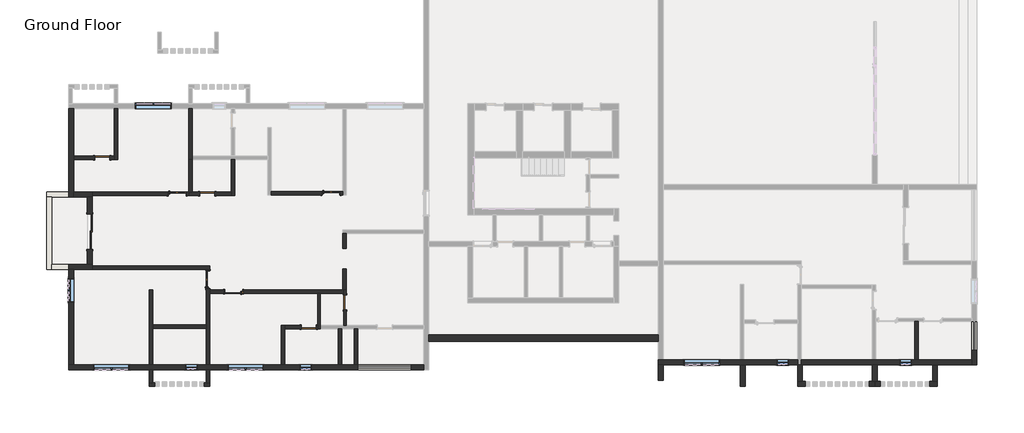
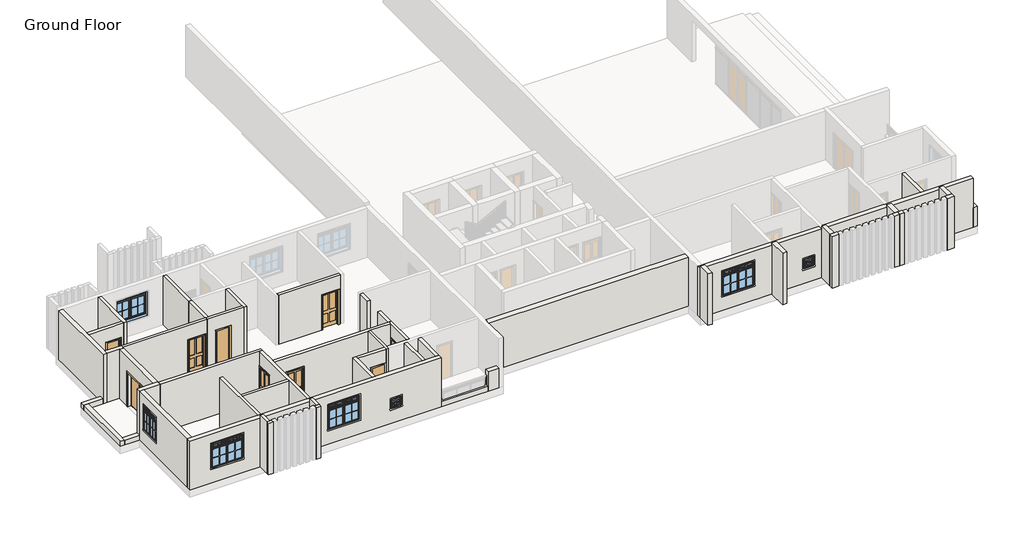
# One storey, part 1 of 9: 51 walls, 9 doors, 9 windows.
"""IFC4 building model written with IfcOpenShell, lengths in millimetres."""

from ifc_helpers import new_model, si_unit, frame, origin, origin_with_axes, place, context, project, spatial, polyline, outline, extrude, faceted_brep, transform, mapped, element, save
from components import door_double_sliding_6_7f701685, door_interior_single_4_panel_wood_3_x_7_bed_room_doors_9f8eaeea, door_0af0cdd0, door_b1104dde, door_6d488673, window_casement_double_awning_double_4_x_5_window_c6f36ef5, window_casement_double_awning_double_6_x_5_2a8633dc, window_double_hung_d0105baa

model = new_model("IFC4")

# Units and contexts
model_context = context("Model", 3, world=origin())
ifc_project = project(units=[si_unit("LENGTHUNIT", "METRE", prefix="MILLI")], contexts=[model_context])

# Site, building, storey
site = spatial("IfcSite", under=ifc_project)
building = spatial("IfcBuilding", under=site)
storey = spatial("IfcBuildingStorey", under=building, Name="Ground Floor", Elevation=0.0)

# Doors
placement = place(None, origin())
door_double_sliding_6_shape = door_double_sliding_6_7f701685(model_context)
element("IfcDoor", 1, ObjectType="Door-Double-Sliding : 6'", at=placement, inside=storey, context=model_context, shape_type="MappedRepresentation", body=[
    mapped(door_double_sliding_6_shape, transform((-13439.7453682, 5075.934892, 0.0), x_axis=(0.0, -1.0, 0.0), y_axis=(1.0, 0.0, 0.0), z_axis=(0.0, 0.0, 1.0))),
])
door_interior_single_4_panel_wood_3_x_7_bed_room_doors_shape = door_interior_single_4_panel_wood_3_x_7_bed_room_doors_9f8eaeea(model_context)
element("IfcDoor", 2, ObjectType="Door-Interior-Single-4_Panel-Wood : 3' x 7' Bed Room Doors", at=placement, inside=storey, context=model_context, shape_type="MappedRepresentation", body=[
    mapped(door_interior_single_4_panel_wood_3_x_7_bed_room_doors_shape, transform((-968.3453682, 7034.909892, 0.0), x_axis=(1.0, 0.0, 0.0), y_axis=(0.0, 1.0, 0.0), z_axis=(0.0, 0.0, 1.0))),
])
element("IfcDoor", 3, ObjectType="Door-Interior-Single-4_Panel-Wood : 3' x 7' Bed Room Doors", at=placement, inside=storey, context=model_context, shape_type="MappedRepresentation", body=[
    mapped(door_interior_single_4_panel_wood_3_x_7_bed_room_doors_shape, transform((-8842.3453682, 7009.509892, 0.0), x_axis=(1.0, 0.0, 0.0), y_axis=(0.0, 1.0, 0.0), z_axis=(0.0, 0.0, 1.0))),
])
element("IfcDoor", 4, ObjectType="Door-Interior-Single-4_Panel-Wood : 3' x 7' Bed Room Doors", at=placement, inside=storey, context=model_context, shape_type="MappedRepresentation", body=[
    mapped(door_interior_single_4_panel_wood_3_x_7_bed_room_doors_shape, transform((-5946.7453682, 1999.359892, 0.0), x_axis=(-1.0, 0.0, 0.0), y_axis=(0.0, -1.0, 0.0), z_axis=(0.0, 0.0, 1.0))),
])
element("IfcDoor", 5, ObjectType="Door-Interior-Single-4_Panel-Wood : 3' x 7' Bed Room Doors", at=placement, inside=storey, context=model_context, shape_type="MappedRepresentation", body=[
    mapped(door_interior_single_4_panel_wood_3_x_7_bed_room_doors_shape, transform((-7258.0203682, 2612.134892, 0.0), x_axis=(0.0, 1.0, 0.0), y_axis=(-1.0, 0.0, 0.0), z_axis=(0.0, 0.0, 1.0))),
])
door_shape = door_0af0cdd0(model_context)
element("IfcDoor", 6, ObjectType="Single-Flush : 30\" x 80\"", at=placement, inside=storey, context=model_context, shape_type="MappedRepresentation", body=[
    mapped(door_shape, transform((-12677.7453682, 8860.534892, 0.0), x_axis=(1.0, 0.0, 0.0), y_axis=(0.0, 1.0, 0.0), z_axis=(0.0, 0.0, 1.0))),
])
door_2_shape = door_b1104dde(model_context)
element("IfcDoor", 7, ObjectType="Single-Flush : 30\" x 80\"", at=placement, inside=storey, context=model_context, shape_type="MappedRepresentation", body=[
    mapped(door_2_shape, transform((-2111.3453682, 173.734892, 0.0), x_axis=(1.0, 0.0, 0.0), y_axis=(0.0, 1.0, 0.0), z_axis=(0.0, 0.0, 1.0))),
])
element("IfcDoor", 8, ObjectType="Single-Flush : 30\" x 80\"", at=placement, inside=storey, context=model_context, shape_type="MappedRepresentation", body=[
    mapped(door_2_shape, transform((-7292.9453682, 7006.334892, 0.0), x_axis=(-1.0, 0.0, 0.0), y_axis=(0.0, -1.0, 0.0), z_axis=(0.0, 0.0, 1.0))),
])
door_3_shape = door_6d488673(model_context)
element("IfcDoor", 9, ObjectType="Single-Flush : 30\" x 80\"", at=placement, inside=storey, context=model_context, shape_type="MappedRepresentation", body=[
    mapped(door_3_shape, transform((-250.7953682, 1456.434892, 0.0), x_axis=(0.0, 1.0, 0.0), y_axis=(-1.0, 0.0, 0.0), z_axis=(0.0, 0.0, 1.0))),
])

# Walls
element("IfcWall", 10, at=placement, inside=storey, context=model_context, shape_type="Brep", body=[
    faceted_brep([(-1654.1453682, 1913.634892, 0.0), (-1654.1453682, 262.634892, 0.0), (-1654.1453682, 84.834892, 0.0), (-1654.1453682, 84.834892, 3048.0), (-1654.1453682, 1913.634892, 3048.0), (-1514.4453682, 84.834892, 0.0), (-1514.4453682, 262.634892, 0.0), (-1514.4453682, 1913.634892, 0.0), (-1514.4453682, 1913.634892, 3048.0), (-1514.4453682, 262.634892, 3048.0), (-1514.4453682, 84.834892, 3048.0)], [[[0, 1, 2, 3, 4]], [[5, 6, 7, 8, 9, 10]], [[2, 1, 0, 7, 6, 5]], [[2, 5, 10, 3]], [[7, 0, 4, 8]], [[4, 3, 10, 9, 8]]]),
])
element("IfcWall", 11, at=placement, inside=storey, context=model_context, shape_type="Brep", body=[
    faceted_brep([(-180.9453682, 1837.434892, 2133.6), (-180.9453682, 1837.434892, 0.0), (-180.9453682, 2091.434892, 0.0), (-180.9453682, 2091.434892, 3048.0), (-180.9453682, 262.634892, 3048.0), (-180.9453682, 262.634892, 0.0), (-180.9453682, 1075.434892, 0.0), (-180.9453682, 1075.434892, 2133.6), (-320.6453682, 1837.434892, 0.0), (-320.6453682, 1837.434892, 2133.6), (-320.6453682, 1075.434892, 2133.6), (-320.6453682, 1075.434892, 0.0), (-320.6453682, 262.634892, 0.0), (-320.6453682, 262.634892, 3048.0), (-320.6453682, 1913.634892, 3048.0), (-320.6453682, 2091.434892, 3048.0), (-320.6453682, 2091.434892, 0.0), (-320.6453682, 1913.634892, 0.0)], [[[0, 1, 2, 3, 4, 5, 6, 7]], [[8, 9, 10, 11, 12, 13, 14, 15, 16, 17]], [[5, 12, 11, 6]], [[16, 2, 1, 8, 17]], [[12, 5, 4, 13]], [[2, 16, 15, 3]], [[4, 3, 15, 14, 13]], [[9, 8, 1, 0]], [[10, 9, 0, 7]], [[11, 10, 7, 6]]]),
])
element("IfcWall", 12, ObjectType="12\" EXTERIOR WALL", at=placement, inside=storey, context=model_context, shape_type="SweptSolid", body=[
    extrude(outline(polyline([(15770.2546318, -550.165108), (4035.4546318, -550.165108), (4035.4546318, -219.965108), (15770.2546318, -219.965108), (15770.2546318, -550.165108)])), origin_with_axes(), (0.0, 0.0, 1.0), 3048.0),
])
element("IfcWall", 13, ObjectType="6\" INTERIOR WALL", at=placement, inside=storey, context=model_context, shape_type="Brep", body=[
    faceted_brep([(-10086.9453682, -1743.965108, 0.0), (-10086.9453682, 110.234892, 0.0), (-10086.9453682, 288.034892, 0.0), (-10086.9453682, 2091.434892, 0.0), (-10086.9453682, 2091.434892, 3048.0), (-10086.9453682, 288.034892, 3048.0), (-10086.9453682, 110.234892, 3048.0), (-10086.9453682, -1743.965108, 3048.0), (-10264.7453682, 2091.434892, 0.0), (-10264.7453682, -1743.965108, 0.0), (-10264.7453682, -1743.965108, 3048.0), (-10264.7453682, 2091.434892, 3048.0)], [[[0, 1, 2, 3, 4, 5, 6, 7]], [[8, 9, 10, 11]], [[3, 2, 1, 0, 9, 8]], [[3, 8, 11, 4]], [[9, 0, 7, 10]], [[7, 6, 5, 4, 11, 10]]]),
])
element("IfcWall", 14, ObjectType="6\" INTERIOR WALL", at=placement, inside=storey, context=model_context, shape_type="Brep", body=[
    faceted_brep([(-7165.9453682, 3094.734892, 0.0), (-7165.9453682, 3132.834892, 0.0), (-7165.9453682, 3132.834892, 3048.0), (-7165.9453682, 2091.434892, 3048.0), (-7165.9453682, 1913.634892, 3048.0), (-7165.9453682, -1743.965108, 3048.0), (-7165.9453682, -1743.965108, 0.0), (-7165.9453682, 1913.634892, 0.0), (-7165.9453682, 2091.434892, 0.0), (-7165.9453682, 2129.534892, 0.0), (-7165.9453682, 2129.534892, 2159.0), (-7165.9453682, 3094.734892, 2159.0), (-7343.7453682, 3132.834892, 0.0), (-7343.7453682, 3094.734892, 0.0), (-7343.7453682, 3094.734892, 2159.0), (-7343.7453682, 2129.534892, 2159.0), (-7343.7453682, 2129.534892, 0.0), (-7343.7453682, 288.034892, 0.0), (-7343.7453682, 110.234892, 0.0), (-7343.7453682, -1743.965108, 0.0), (-7343.7453682, -1743.965108, 3048.0), (-7343.7453682, 110.234892, 3048.0), (-7343.7453682, 288.034892, 3048.0), (-7343.7453682, 3132.834892, 3048.0)], [[[0, 1, 2, 3, 4, 5, 6, 7, 8, 9, 10, 11]], [[12, 13, 14, 15, 16, 17, 18, 19, 20, 21, 22, 23]], [[6, 19, 18, 17, 16, 9, 8, 7]], [[12, 1, 0, 13]], [[19, 6, 5, 20]], [[5, 4, 3, 2, 23, 22, 21, 20]], [[1, 12, 23, 2]], [[11, 14, 13, 0]], [[14, 11, 10, 15]], [[15, 10, 9, 16]]]),
])
element("IfcWall", 15, ObjectType="6\" INTERIOR WALL", at=placement, inside=storey, context=model_context, shape_type="SweptSolid", body=[
    extrude(outline(polyline([(-10086.9453682, 288.034892), (-7343.7453682, 288.034892), (-7343.7453682, 110.234892), (-10086.9453682, 110.234892), (-10086.9453682, 288.034892)])), origin_with_axes(), (0.0, 0.0, 1.0), 3048.0),
])
element("IfcWall", 16, ObjectType="6\" INTERIOR WALL", at=placement, inside=storey, context=model_context, shape_type="Brep", body=[
    faceted_brep([(-3330.5453682, -1743.965108, 0.0), (-3330.5453682, 84.834892, 0.0), (-3330.5453682, 262.634892, 0.0), (-3330.5453682, 262.634892, 3048.0), (-3330.5453682, 84.834892, 3048.0), (-3330.5453682, -1743.965108, 3048.0), (-3508.3453682, 262.634892, 0.0), (-3508.3453682, -1743.965108, 0.0), (-3508.3453682, -1743.965108, 3048.0), (-3508.3453682, 262.634892, 3048.0)], [[[0, 1, 2, 3, 4, 5]], [[6, 7, 8, 9]], [[2, 1, 0, 7, 6]], [[7, 0, 5, 8]], [[2, 6, 9, 3]], [[5, 4, 3, 9, 8]]]),
])
element("IfcWall", 17, ObjectType="6\" INTERIOR WALL", at=placement, inside=storey, context=model_context, shape_type="Brep", body=[
    faceted_brep([(-6429.3453682, 2091.434892, 0.0), (-7165.9453682, 2091.434892, 0.0), (-7165.9453682, 2091.434892, 3048.0), (-358.7453682, 2091.434892, 3048.0), (-320.6453682, 2091.434892, 3048.0), (-320.6453682, 2091.434892, 0.0), (-358.7453682, 2091.434892, 0.0), (-5464.1453682, 2091.434892, 0.0), (-5464.1453682, 2091.434892, 2159.0), (-6429.3453682, 2091.434892, 2159.0), (-7165.9453682, 1913.634892, 0.0), (-6429.3453682, 1913.634892, 0.0), (-6429.3453682, 1913.634892, 2159.0), (-5464.1453682, 1913.634892, 2159.0), (-5464.1453682, 1913.634892, 0.0), (-1654.1453682, 1913.634892, 0.0), (-1514.4453682, 1913.634892, 0.0), (-320.6453682, 1913.634892, 0.0), (-320.6453682, 1913.634892, 3048.0), (-1514.4453682, 1913.634892, 3048.0), (-1654.1453682, 1913.634892, 3048.0), (-7165.9453682, 1913.634892, 3048.0)], [[[0, 1, 2, 3, 4, 5, 6, 7, 8, 9]], [[10, 11, 12, 13, 14, 15, 16, 17, 18, 19, 20, 21]], [[5, 17, 16, 15, 14, 7, 6]], [[10, 1, 0, 11]], [[17, 5, 4, 18]], [[1, 10, 21, 2]], [[4, 3, 2, 21, 20, 19, 18]], [[9, 12, 11, 0]], [[12, 9, 8, 13]], [[13, 8, 7, 14]]]),
])
element("IfcWall", 18, ObjectType="6\" INTERIOR WALL", at=placement, inside=storey, context=model_context, shape_type="SweptSolid", body=[
    extrude(outline(polyline([(2133.6, -1730.3453682), (0.0, -1730.3453682), (0.0, -1654.1453682), (3048.0, -1654.1453682), (3048.0, -3330.5453682), (0.0, -3330.5453682), (0.0, -2492.3453682), (2133.6, -2492.3453682), (2133.6, -1730.3453682)])), frame((0.0, 84.834892, 0.0), z_axis=(0.0, 1.0, 0.0), x_axis=(0.0, 0.0, 1.0)), (0.0, 0.0, 1.0), 177.8),
])
element("IfcWall", 19, ObjectType="6\" INTERIOR WALL", at=placement, inside=storey, context=model_context, shape_type="SweptSolid", body=[
    extrude(outline(polyline([(-409.5453682, 84.834892), (-409.5453682, -1743.965108), (-587.3453682, -1743.965108), (-587.3453682, 84.834892), (-409.5453682, 84.834892)])), origin_with_axes(), (0.0, 0.0, 1.0), 3048.0),
])
element("IfcWall", 20, ObjectType="6\" INTERIOR WALL", at=placement, inside=storey, context=model_context, shape_type="SweptSolid", body=[
    extrude(outline(polyline([(-358.7453682, 4225.034892), (-358.7453682, 4987.034892), (-180.9453682, 4987.034892), (-180.9453682, 4225.034892), (-358.7453682, 4225.034892)])), origin_with_axes(), (0.0, 0.0, 1.0), 3048.0),
])
element("IfcWall", 21, ObjectType="6\" INTERIOR WALL", at=placement, inside=storey, context=model_context, shape_type="Brep", body=[
    faceted_brep([(-358.7453682, 3158.234892, 0.0), (-358.7453682, 2091.434892, 0.0), (-358.7453682, 2091.434892, 3048.0), (-358.7453682, 3158.234892, 3048.0), (-180.9453682, 2091.434892, 0.0), (-180.9453682, 3158.234892, 0.0), (-180.9453682, 3158.234892, 3048.0), (-180.9453682, 2091.434892, 3048.0), (-320.6453682, 2091.434892, 0.0), (-320.6453682, 2091.434892, 3048.0)], [[[0, 1, 2, 3]], [[4, 5, 6, 7]], [[1, 0, 5, 4, 8]], [[5, 0, 3, 6]], [[1, 8, 4, 7, 9, 2]], [[3, 2, 9, 7, 6]]]),
])
element("IfcWall", 22, ObjectType="6\" INTERIOR WALL", at=placement, inside=storey, context=model_context, shape_type="SweptSolid", body=[
    extrude(outline(polyline([(0.0, -485.7453682), (0.0, -358.7453682), (3048.0, -358.7453682), (3048.0, -4016.3453682), (0.0, -4016.3453682), (0.0, -1450.9453682), (2159.0, -1450.9453682), (2159.0, -485.7453682), (0.0, -485.7453682)])), frame((0.0, 6942.834892, 0.0), z_axis=(0.0, 1.0, 0.0), x_axis=(0.0, 0.0, 1.0)), (0.0, 0.0, 1.0), 177.8),
])
element("IfcWall", 23, ObjectType="6\" INTERIOR WALL", at=placement, inside=storey, context=model_context, shape_type="Brep", body=[
    faceted_brep([(-8232.7453682, 11387.834892, 0.0), (-8232.7453682, 8771.634892, 0.0), (-8232.7453682, 8771.634892, 3048.0), (-8232.7453682, 11387.834892, 3048.0), (-8054.9453682, 8771.634892, 0.0), (-8054.9453682, 8949.434892, 0.0), (-8054.9453682, 11387.834892, 0.0), (-8054.9453682, 11387.834892, 3048.0), (-8054.9453682, 8949.434892, 3048.0), (-8054.9453682, 8771.634892, 3048.0)], [[[0, 1, 2, 3]], [[4, 5, 6, 7, 8, 9]], [[1, 0, 6, 5, 4]], [[6, 0, 3, 7]], [[1, 4, 9, 2]], [[3, 2, 9, 8, 7]]]),
])
element("IfcWall", 24, ObjectType="6\" INTERIOR WALL", at=placement, inside=storey, context=model_context, shape_type="Brep", body=[
    faceted_brep([(-6073.7453682, 8771.634892, 0.0), (-6073.7453682, 7095.234892, 0.0), (-6073.7453682, 6917.434892, 0.0), (-6073.7453682, 6917.434892, 3048.0), (-6073.7453682, 8771.634892, 3048.0), (-5895.9453682, 6917.434892, 0.0), (-5895.9453682, 8771.634892, 0.0), (-5895.9453682, 8771.634892, 3048.0), (-5895.9453682, 6917.434892, 3048.0)], [[[0, 1, 2, 3, 4]], [[5, 6, 7, 8]], [[2, 1, 0, 6, 5]], [[6, 0, 4, 7]], [[2, 5, 8, 3]], [[4, 3, 8, 7]]]),
])
element("IfcWall", 25, ObjectType="6\" INTERIOR WALL", at=placement, inside=storey, context=model_context, shape_type="Brep", body=[
    faceted_brep([(-7673.9453682, 7095.234892, 2133.6), (-7673.9453682, 7095.234892, 0.0), (-8054.9453682, 7095.234892, 0.0), (-8232.7453682, 7095.234892, 0.0), (-8232.7453682, 7095.234892, 3048.0), (-8054.9453682, 7095.234892, 3048.0), (-6073.7453682, 7095.234892, 3048.0), (-6073.7453682, 7095.234892, 0.0), (-6911.9453682, 7095.234892, 0.0), (-6911.9453682, 7095.234892, 2133.6), (-7673.9453682, 6917.434892, 0.0), (-7673.9453682, 6917.434892, 2133.6), (-6911.9453682, 6917.434892, 2133.6), (-6911.9453682, 6917.434892, 0.0), (-6073.7453682, 6917.434892, 0.0), (-6073.7453682, 6917.434892, 3048.0), (-8232.7453682, 6917.434892, 3048.0), (-8232.7453682, 6917.434892, 0.0)], [[[0, 1, 2, 3, 4, 5, 6, 7, 8, 9]], [[10, 11, 12, 13, 14, 15, 16, 17]], [[7, 14, 13, 8]], [[17, 3, 2, 1, 10]], [[14, 7, 6, 15]], [[3, 17, 16, 4]], [[6, 5, 4, 16, 15]], [[11, 10, 1, 0]], [[12, 11, 0, 9]], [[13, 12, 9, 8]]]),
])
element("IfcWall", 26, ObjectType="6\" INTERIOR WALL", at=placement, inside=storey, context=model_context, shape_type="SweptSolid", body=[
    extrude(outline(polyline([(-8054.9453682, 8771.634892), (-8054.9453682, 7095.234892), (-8232.7453682, 7095.234892), (-8232.7453682, 8771.634892), (-8054.9453682, 8771.634892)])), origin_with_axes(), (0.0, 0.0, 1.0), 3048.0),
])
element("IfcWall", 27, ObjectType="6\" INTERIOR WALL", at=placement, inside=storey, context=model_context, shape_type="Brep", body=[
    faceted_brep([(-12068.1453682, 11387.834892, 0.0), (-12068.1453682, 8949.434892, 0.0), (-12068.1453682, 8771.634892, 0.0), (-12068.1453682, 8771.634892, 3048.0), (-12068.1453682, 8949.434892, 3048.0), (-12068.1453682, 11387.834892, 3048.0), (-11890.3453682, 8771.634892, 0.0), (-11890.3453682, 11387.834892, 0.0), (-11890.3453682, 11387.834892, 3048.0), (-11890.3453682, 8771.634892, 3048.0)], [[[0, 1, 2, 3, 4, 5]], [[6, 7, 8, 9]], [[2, 1, 0, 7, 6]], [[7, 0, 5, 8]], [[2, 6, 9, 3]], [[5, 4, 3, 9, 8]]]),
])
element("IfcWall", 28, ObjectType="6\" INTERIOR WALL", at=placement, inside=storey, context=model_context, shape_type="SweptSolid", body=[
    extrude(outline(polyline([(2133.6, -12296.7453682), (0.0, -12296.7453682), (0.0, -12068.1453682), (3048.0, -12068.1453682), (3048.0, -14138.2453682), (0.0, -14138.2453682), (0.0, -13058.7453682), (2133.6, -13058.7453682), (2133.6, -12296.7453682)])), frame((0.0, 8771.634892, 0.0), z_axis=(0.0, 1.0, 0.0), x_axis=(0.0, 0.0, 1.0)), (0.0, 0.0, 1.0), 177.8),
])
element("IfcWall", 29, ObjectType="6\" INTERIOR WALL", at=placement, inside=storey, context=model_context, shape_type="SweptSolid", body=[
    extrude(outline(polyline([(403.2546318, 84.834892), (403.2546318, -1743.965108), (225.4546318, -1743.965108), (225.4546318, 84.834892), (403.2546318, 84.834892)])), origin_with_axes(), (0.0, 0.0, 1.0), 3048.0),
])
element("IfcWall", 30, ObjectType="6\" INTERIOR WALL", at=placement, inside=storey, context=model_context, shape_type="Brep", body=[
    faceted_brep([(-13185.7453682, 3132.834892, 0.0), (-7343.7453682, 3132.834892, 0.0), (-7165.9453682, 3132.834892, 0.0), (-7165.9453682, 3132.834892, 3048.0), (-7343.7453682, 3132.834892, 3048.0), (-13185.7453682, 3132.834892, 3048.0), (-7165.9453682, 3310.634892, 0.0), (-13185.7453682, 3310.634892, 0.0), (-13185.7453682, 3310.634892, 3048.0), (-7165.9453682, 3310.634892, 3048.0)], [[[0, 1, 2, 3, 4, 5]], [[6, 7, 8, 9]], [[2, 1, 0, 7, 6]], [[7, 0, 5, 8]], [[5, 4, 3, 9, 8]], [[2, 6, 9, 3]]]),
])
element("IfcWall", 31, ObjectType="6\" INTERIOR WALL", at=placement, inside=storey, context=model_context, shape_type="SweptSolid", body=[
    extrude(outline(polyline([(0.0, -8359.7453682), (0.0, -8232.7453682), (3048.0, -8232.7453682), (3048.0, -13185.7453682), (0.0, -13185.7453682), (0.0, -9324.9453682), (2159.0, -9324.9453682), (2159.0, -8359.7453682), (0.0, -8359.7453682)])), frame((0.0, 6917.434892, 0.0), z_axis=(0.0, 1.0, 0.0), x_axis=(0.0, 0.0, 1.0)), (0.0, 0.0, 1.0), 177.8),
])
element("IfcWall", 32, ObjectType="6\" INTERIOR WALL", at=placement, inside=storey, context=model_context, shape_type="SweptSolid", body=[
    extrude(outline(polyline([(29079.8546318, 465.834892), (29079.8546318, -1489.965108), (28902.0546318, -1489.965108), (28902.0546318, 465.834892), (29079.8546318, 465.834892)])), origin_with_axes(), (0.0, 0.0, 1.0), 3048.0),
])
element("IfcWall", 33, ObjectType="6\" INTERIOR WALL", at=placement, inside=storey, context=model_context, shape_type="SweptSolid", body=[
    extrude(outline(polyline([(-10264.7453682, -2658.365108), (-10264.7453682, -1997.965108), (-10086.9453682, -1997.965108), (-10086.9453682, -2658.365108), (-10264.7453682, -2658.365108)])), origin_with_axes(), (0.0, 0.0, 1.0), 3200.4),
])
element("IfcWall", 34, ObjectType="6\" INTERIOR WALL", at=placement, inside=storey, context=model_context, shape_type="SweptSolid", body=[
    extrude(outline(polyline([(-7343.7453682, -2658.365108), (-7343.7453682, -1997.965108), (-7165.9453682, -1997.965108), (-7165.9453682, -2658.365108), (-7343.7453682, -2658.365108)])), origin_with_axes(), (0.0, 0.0, 1.0), 3200.4),
])
element("IfcWall", 35, ObjectType="6\" INTERIOR WALL", at=placement, inside=storey, context=model_context, shape_type="Brep", body=[
    faceted_brep([(-10264.7453682, -2836.165108, 0.0), (-9972.6453682, -2836.165108, 0.0), (-9972.6453682, -2836.165108, 3200.4), (-10264.7453682, -2836.165108, 3200.4), (-10264.7453682, -2658.365108, 0.0), (-10264.7453682, -2658.365108, 3200.4), (-10086.9453682, -2658.365108, 3200.4), (-9972.6453682, -2658.365108, 3200.4), (-9972.6453682, -2658.365108, 0.0), (-10086.9453682, -2658.365108, 0.0)], [[[0, 1, 2, 3]], [[4, 5, 6, 7, 8, 9]], [[1, 0, 4, 9, 8]], [[2, 1, 8, 7]], [[3, 2, 7, 6, 5]], [[0, 3, 5, 4]]]),
])
element("IfcWall", 36, ObjectType="6\" INTERIOR WALL", at=placement, inside=storey, context=model_context, shape_type="Brep", body=[
    faceted_brep([(-7165.9453682, -2658.365108, 0.0), (-7343.7453682, -2658.365108, 0.0), (-7458.0453682, -2658.365108, 0.0), (-7458.0453682, -2658.365108, 3200.4), (-7343.7453682, -2658.365108, 3200.4), (-7165.9453682, -2658.365108, 3200.4), (-7165.9453682, -2836.165108, 0.0), (-7165.9453682, -2836.165108, 3200.4), (-7458.0453682, -2836.165108, 3200.4), (-7458.0453682, -2836.165108, 0.0)], [[[0, 1, 2, 3, 4, 5]], [[6, 7, 8, 9]], [[2, 1, 0, 6, 9]], [[3, 2, 9, 8]], [[5, 4, 3, 8, 7]], [[0, 5, 7, 6]]]),
])
element("IfcWall", 37, ObjectType="9\" EXTERIOR WALL", at=placement, inside=storey, context=model_context, shape_type="Brep", body=[
    faceted_brep([(-14392.2453682, -1997.965108, 0.0), (-10264.7453682, -1997.965108, 0.0), (-10086.9453682, -1997.965108, 0.0), (-7343.7453682, -1997.965108, 0.0), (-7165.9453682, -1997.965108, 0.0), (403.2546318, -1997.965108, 0.0), (403.2546318, -1997.965108, 304.8), (403.2546318, -1997.965108, 3048.0), (-14392.2453682, -1997.965108, 3048.0), (-13115.8953682, -1997.965108, 914.4), (-13115.8953682, -1997.965108, 2438.4), (-11287.0953682, -1997.965108, 2438.4), (-11287.0953682, -1997.965108, 914.4), (-6251.5453682, -1997.965108, 914.4), (-6251.5453682, -1997.965108, 2438.4), (-4422.7453682, -1997.965108, 2438.4), (-4422.7453682, -1997.965108, 914.4), (-7800.9453682, -1997.965108, 1524.0), (-7800.9453682, -1997.965108, 914.4), (-8410.5453682, -1997.965108, 914.4), (-8410.5453682, -1997.965108, 1524.0), (-1958.9453682, -1997.965108, 1524.0), (-1958.9453682, -1997.965108, 914.4), (-2568.5453682, -1997.965108, 914.4), (-2568.5453682, -1997.965108, 1524.0), (403.2546318, -1743.965108, 0.0), (225.4546318, -1743.965108, 0.0), (-409.5453682, -1743.965108, 0.0), (-587.3453682, -1743.965108, 0.0), (-3330.5453682, -1743.965108, 0.0), (-3508.3453682, -1743.965108, 0.0), (-7165.9453682, -1743.965108, 0.0), (-7343.7453682, -1743.965108, 0.0), (-10086.9453682, -1743.965108, 0.0), (-10264.7453682, -1743.965108, 0.0), (-14138.2453682, -1743.965108, 0.0), (-14392.2453682, -1743.965108, 0.0), (-14392.2453682, -1743.965108, 3048.0), (-14138.2453682, -1743.965108, 3048.0), (-10264.7453682, -1743.965108, 3048.0), (-10086.9453682, -1743.965108, 3048.0), (-7343.7453682, -1743.965108, 3048.0), (-7165.9453682, -1743.965108, 3048.0), (-3508.3453682, -1743.965108, 3048.0), (-3330.5453682, -1743.965108, 3048.0), (-587.3453682, -1743.965108, 3048.0), (-409.5453682, -1743.965108, 3048.0), (225.4546318, -1743.965108, 3048.0), (403.2546318, -1743.965108, 3048.0), (403.2546318, -1743.965108, 304.8), (-13115.8953682, -1743.965108, 2438.4), (-13115.8953682, -1743.965108, 914.4), (-11287.0953682, -1743.965108, 914.4), (-11287.0953682, -1743.965108, 2438.4), (-6251.5453682, -1743.965108, 2438.4), (-6251.5453682, -1743.965108, 914.4), (-4422.7453682, -1743.965108, 914.4), (-4422.7453682, -1743.965108, 2438.4), (-7800.9453682, -1743.965108, 914.4), (-7800.9453682, -1743.965108, 1524.0), (-8410.5453682, -1743.965108, 1524.0), (-8410.5453682, -1743.965108, 914.4), (-1958.9453682, -1743.965108, 914.4), (-1958.9453682, -1743.965108, 1524.0), (-2568.5453682, -1743.965108, 1524.0), (-2568.5453682, -1743.965108, 914.4)], [[[0, 1, 2, 3, 4, 5, 6, 7, 8], [9, 10, 11, 12], [13, 14, 15, 16], [17, 18, 19, 20], [21, 22, 23, 24]], [[25, 26, 27, 28, 29, 30, 31, 32, 33, 34, 35, 36, 37, 38, 39, 40, 41, 42, 43, 44, 45, 46, 47, 48, 49], [50, 51, 52, 53], [54, 55, 56, 57], [58, 59, 60, 61], [62, 63, 64, 65]], [[5, 4, 3, 2, 1, 0, 36, 35, 34, 33, 32, 31, 30, 29, 28, 27, 26, 25]], [[5, 25, 49, 48, 7, 6]], [[36, 0, 8, 37]], [[8, 7, 48, 47, 46, 45, 44, 43, 42, 41, 40, 39, 38, 37]], [[51, 50, 10, 9]], [[52, 51, 9, 12]], [[53, 52, 12, 11]], [[50, 53, 11, 10]], [[55, 54, 14, 13]], [[56, 55, 13, 16]], [[57, 56, 16, 15]], [[54, 57, 15, 14]], [[18, 17, 59, 58]], [[19, 18, 58, 61]], [[20, 19, 61, 60]], [[17, 20, 60, 59]], [[22, 21, 63, 62]], [[23, 22, 62, 65]], [[24, 23, 65, 64]], [[21, 24, 64, 63]]]),
])
element("IfcWall", 38, ObjectType="9\" EXTERIOR WALL", at=placement, inside=storey, context=model_context, shape_type="SweptSolid", body=[
    extrude(outline(polyline([(3132.834892, 0.0), (-1743.965108, 0.0), (-1743.965108, 3048.0), (3132.834892, 3048.0), (3132.834892, 0.0)]), holes=[polyline([(2675.634892, 914.4), (2675.634892, 2438.4), (1456.434892, 2438.4), (1456.434892, 914.4), (2675.634892, 914.4)])]), frame((-14392.2453682, 0.0, 0.0), z_axis=(1.0, 0.0, 0.0), x_axis=(0.0, 1.0, 0.0)), (0.0, 0.0, 1.0), 254.0),
])
element("IfcWall", 39, ObjectType="9\" EXTERIOR WALL", at=placement, inside=storey, context=model_context, shape_type="SweptSolid", body=[
    extrude(outline(polyline([(-14392.2453682, 3132.834892), (-15268.5453682, 3132.834892), (-15268.5453682, 3386.834892), (-14392.2453682, 3386.834892), (-14392.2453682, 3132.834892)])), origin_with_axes(), (0.0, 0.0, 1.0), 304.8),
])
element("IfcWall", 40, ObjectType="9\" EXTERIOR WALL", at=placement, inside=storey, context=model_context, shape_type="Brep", body=[
    faceted_brep([(-14392.2453682, 11387.834892, 0.0), (-14392.2453682, 7095.234892, 0.0), (-14392.2453682, 6841.234892, 0.0), (-14392.2453682, 6841.234892, 304.8), (-14392.2453682, 6841.234892, 3048.0), (-14392.2453682, 11387.834892, 3048.0), (-14138.2453682, 6841.234892, 0.0), (-14138.2453682, 7095.234892, 0.0), (-14138.2453682, 8771.634892, 0.0), (-14138.2453682, 8949.434892, 0.0), (-14138.2453682, 11387.834892, 0.0), (-14138.2453682, 11387.834892, 3048.0), (-14138.2453682, 8949.434892, 3048.0), (-14138.2453682, 8771.634892, 3048.0), (-14138.2453682, 7095.234892, 3048.0), (-14138.2453682, 6841.234892, 3048.0)], [[[0, 1, 2, 3, 4, 5]], [[6, 7, 8, 9, 10, 11, 12, 13, 14, 15]], [[2, 1, 0, 10, 9, 8, 7, 6]], [[10, 0, 5, 11]], [[2, 6, 15, 4, 3]], [[5, 4, 15, 14, 13, 12, 11]]]),
])
element("IfcWall", 41, ObjectType="9\" EXTERIOR WALL", at=placement, inside=storey, context=model_context, shape_type="Brep", body=[
    faceted_brep([(-14138.2453682, 6841.234892, 0.0), (-13439.7453682, 6841.234892, 0.0), (-13185.7453682, 6841.234892, 0.0), (-13185.7453682, 6841.234892, 3048.0), (-13439.7453682, 6841.234892, 3048.0), (-14138.2453682, 6841.234892, 3048.0), (-13185.7453682, 7095.234892, 0.0), (-14138.2453682, 7095.234892, 0.0), (-14138.2453682, 7095.234892, 3048.0), (-13185.7453682, 7095.234892, 3048.0), (-13185.7453682, 6917.434892, 0.0), (-13185.7453682, 6917.434892, 3048.0)], [[[0, 1, 2, 3, 4, 5]], [[6, 7, 8, 9]], [[2, 1, 0, 7, 6, 10]], [[2, 10, 6, 9, 11, 3]], [[7, 0, 5, 8]], [[5, 4, 3, 11, 9, 8]]]),
])
element("IfcWall", 42, ObjectType="9\" EXTERIOR WALL", at=placement, inside=storey, context=model_context, shape_type="SweptSolid", body=[
    extrude(outline(polyline([(5990.334892, 0.0), (5990.334892, 2133.6), (4161.534892, 2133.6), (4161.534892, 0.0), (3386.834892, 0.0), (3386.834892, 3048.0), (6841.234892, 3048.0), (6841.234892, 0.0), (5990.334892, 0.0)])), frame((-13439.7453682, 0.0, 0.0), z_axis=(1.0, 0.0, 0.0), x_axis=(0.0, 1.0, 0.0)), (0.0, 0.0, 1.0), 254.0),
])
element("IfcWall", 43, ObjectType="9\" EXTERIOR WALL", at=placement, inside=storey, context=model_context, shape_type="Brep", body=[
    faceted_brep([(-14392.2453682, 7095.234892, 0.0), (-15522.5453682, 7095.234892, 0.0), (-15522.5453682, 7095.234892, 304.8), (-14392.2453682, 7095.234892, 304.8), (-14392.2453682, 6841.234892, 0.0), (-14392.2453682, 6841.234892, 304.8), (-15268.5453682, 6841.234892, 304.8), (-15522.5453682, 6841.234892, 304.8), (-15522.5453682, 6841.234892, 0.0), (-15268.5453682, 6841.234892, 0.0)], [[[0, 1, 2, 3]], [[4, 5, 6, 7, 8, 9]], [[1, 0, 4, 9, 8]], [[3, 2, 7, 6, 5]], [[0, 3, 5, 4]], [[2, 1, 8, 7]]]),
])
element("IfcWall", 44, ObjectType="9\" EXTERIOR WALL", at=placement, inside=storey, context=model_context, shape_type="Brep", body=[
    faceted_brep([(-15522.5453682, 6841.234892, 0.0), (-15522.5453682, 3132.834892, 0.0), (-15522.5453682, 3132.834892, 304.8), (-15522.5453682, 6841.234892, 304.8), (-15268.5453682, 6841.234892, 0.0), (-15268.5453682, 6841.234892, 304.8), (-15268.5453682, 3386.834892, 304.8), (-15268.5453682, 3132.834892, 304.8), (-15268.5453682, 3132.834892, 0.0), (-15268.5453682, 3386.834892, 0.0)], [[[0, 1, 2, 3]], [[4, 5, 6, 7, 8, 9]], [[1, 0, 4, 9, 8]], [[3, 2, 7, 6, 5]], [[0, 3, 5, 4]], [[2, 1, 8, 7]]]),
])
element("IfcWall", 45, ObjectType="9\" EXTERIOR WALL", at=placement, inside=storey, context=model_context, shape_type="Brep", body=[
    faceted_brep([(22907.6546318, -1489.965108, 0.0), (20164.4546318, -1489.965108, 0.0), (19986.6546318, -1489.965108, 0.0), (16024.2546318, -1489.965108, 0.0), (15770.2546318, -1489.965108, 0.0), (15770.2546318, -1489.965108, 3048.0), (16024.2546318, -1489.965108, 3048.0), (19986.6546318, -1489.965108, 3048.0), (20164.4546318, -1489.965108, 3048.0), (22907.6546318, -1489.965108, 3048.0), (17091.0546318, -1489.965108, 2438.4), (17091.0546318, -1489.965108, 914.4), (18919.8546318, -1489.965108, 914.4), (18919.8546318, -1489.965108, 2438.4), (22450.4546318, -1489.965108, 914.4), (22450.4546318, -1489.965108, 1524.0), (21840.8546318, -1489.965108, 1524.0), (21840.8546318, -1489.965108, 914.4), (15770.2546318, -1743.965108, 0.0), (16024.2546318, -1743.965108, 0.0), (19986.6546318, -1743.965108, 0.0), (20240.6546318, -1743.965108, 0.0), (22907.6546318, -1743.965108, 0.0), (22907.6546318, -1743.965108, 3048.0), (15770.2546318, -1743.965108, 3048.0), (17091.0546318, -1743.965108, 914.4), (17091.0546318, -1743.965108, 2438.4), (18919.8546318, -1743.965108, 2438.4), (18919.8546318, -1743.965108, 914.4), (22450.4546318, -1743.965108, 1524.0), (22450.4546318, -1743.965108, 914.4), (21840.8546318, -1743.965108, 914.4), (21840.8546318, -1743.965108, 1524.0)], [[[0, 1, 2, 3, 4, 5, 6, 7, 8, 9], [10, 11, 12, 13], [14, 15, 16, 17]], [[18, 19, 20, 21, 22, 23, 24], [25, 26, 27, 28], [29, 30, 31, 32]], [[4, 3, 2, 1, 0, 22, 21, 20, 19, 18]], [[22, 0, 9, 23]], [[9, 8, 7, 6, 5, 24, 23]], [[11, 10, 26, 25]], [[12, 11, 25, 28]], [[13, 12, 28, 27]], [[10, 13, 27, 26]], [[30, 29, 15, 14]], [[31, 30, 14, 17]], [[32, 31, 17, 16]], [[29, 32, 16, 15]], [[4, 18, 24, 5]]]),
])
element("IfcWall", 46, ObjectType="9\" EXTERIOR WALL", at=placement, inside=storey, context=model_context, shape_type="Brep", body=[
    faceted_brep([(23085.4546318, -1743.965108, 0.0), (23161.6546318, -1743.965108, 0.0), (26743.0546318, -1743.965108, 0.0), (26997.0546318, -1743.965108, 0.0), (29816.4546318, -1743.965108, 0.0), (30070.4546318, -1743.965108, 0.0), (31823.0546318, -1743.965108, 0.0), (31823.0546318, -1743.965108, 1219.2), (31823.0546318, -1743.965108, 3048.0), (23085.4546318, -1743.965108, 3048.0), (28749.6546318, -1743.965108, 1524.0), (28749.6546318, -1743.965108, 914.4), (28140.0546318, -1743.965108, 914.4), (28140.0546318, -1743.965108, 1524.0), (31823.0546318, -1489.965108, 0.0), (29079.8546318, -1489.965108, 0.0), (28902.0546318, -1489.965108, 0.0), (26920.8546318, -1489.965108, 0.0), (26743.0546318, -1489.965108, 0.0), (23085.4546318, -1489.965108, 0.0), (23085.4546318, -1489.965108, 3048.0), (26743.0546318, -1489.965108, 3048.0), (26920.8546318, -1489.965108, 3048.0), (28902.0546318, -1489.965108, 3048.0), (29079.8546318, -1489.965108, 3048.0), (31823.0546318, -1489.965108, 3048.0), (28749.6546318, -1489.965108, 914.4), (28749.6546318, -1489.965108, 1524.0), (28140.0546318, -1489.965108, 1524.0), (28140.0546318, -1489.965108, 914.4)], [[[0, 1, 2, 3, 4, 5, 6, 7, 8, 9], [10, 11, 12, 13]], [[14, 15, 16, 17, 18, 19, 20, 21, 22, 23, 24, 25], [26, 27, 28, 29]], [[6, 5, 4, 3, 2, 1, 0, 19, 18, 17, 16, 15, 14]], [[19, 0, 9, 20]], [[9, 8, 25, 24, 23, 22, 21, 20]], [[11, 10, 27, 26]], [[12, 11, 26, 29]], [[13, 12, 29, 28]], [[10, 13, 28, 27]], [[6, 14, 25, 8, 7]]]),
])
element("IfcWall", 47, ObjectType="9\" EXTERIOR WALL", at=placement, inside=storey, context=model_context, shape_type="Brep", body=[
    faceted_brep([(-14392.2453682, 3132.834892, 0.0), (-14138.2453682, 3132.834892, 0.0), (-13185.7453682, 3132.834892, 0.0), (-13185.7453682, 3132.834892, 3048.0), (-14138.2453682, 3132.834892, 3048.0), (-14392.2453682, 3132.834892, 3048.0), (-14392.2453682, 3132.834892, 304.8), (-13185.7453682, 3386.834892, 0.0), (-13439.7453682, 3386.834892, 0.0), (-14392.2453682, 3386.834892, 0.0), (-14392.2453682, 3386.834892, 304.8), (-14392.2453682, 3386.834892, 3048.0), (-13439.7453682, 3386.834892, 3048.0), (-13185.7453682, 3386.834892, 3048.0), (-13185.7453682, 3310.634892, 0.0), (-13185.7453682, 3310.634892, 3048.0)], [[[0, 1, 2, 3, 4, 5, 6]], [[7, 8, 9, 10, 11, 12, 13]], [[2, 1, 0, 9, 8, 7, 14]], [[9, 0, 6, 5, 11, 10]], [[2, 14, 7, 13, 15, 3]], [[5, 4, 3, 15, 13, 12, 11]]]),
])
element("IfcWall", 48, ObjectType="9\" EXTERIOR WALL", at=placement, inside=storey, context=model_context, shape_type="SweptSolid", body=[
    extrude(outline(polyline([(3146.4546318, -1997.965108), (403.2546318, -1997.965108), (403.2546318, -1743.965108), (3146.4546318, -1743.965108), (3146.4546318, -1997.965108)])), origin_with_axes(), (0.0, 0.0, 1.0), 304.8),
])
element("IfcWall", 49, ObjectType="9\" EXTERIOR WALL", at=placement, inside=storey, context=model_context, shape_type="Brep", body=[
    faceted_brep([(3146.4546318, -1997.965108, 0.0), (3781.4546318, -1997.965108, 0.0), (3781.4546318, -1997.965108, 1219.2), (3146.4546318, -1997.965108, 1219.2), (3146.4546318, -1997.965108, 304.8), (3146.4546318, -1743.965108, 0.0), (3146.4546318, -1743.965108, 304.8), (3146.4546318, -1743.965108, 1219.2), (3781.4546318, -1743.965108, 1219.2), (3781.4546318, -1743.965108, 0.0)], [[[0, 1, 2, 3, 4]], [[5, 6, 7, 8, 9]], [[1, 0, 5, 9]], [[3, 2, 8, 7]], [[0, 4, 3, 7, 6, 5]], [[2, 1, 9, 8]]]),
])
element("IfcWall", 50, ObjectType="9\" EXTERIOR WALL", at=placement, inside=storey, context=model_context, shape_type="SweptSolid", body=[
    extrude(outline(polyline([(32077.0546318, 465.834892), (32077.0546318, -1007.365108), (31823.0546318, -1007.365108), (31823.0546318, 465.834892), (32077.0546318, 465.834892)])), origin_with_axes(), (0.0, 0.0, 1.0), 304.8),
])
element("IfcWall", 51, ObjectType="9\" EXTERIOR WALL", at=placement, inside=storey, context=model_context, shape_type="Brep", body=[
    faceted_brep([(32077.0546318, -1743.965108, 0.0), (32077.0546318, -1007.365108, 0.0), (32077.0546318, -1007.365108, 304.8), (32077.0546318, -1007.365108, 1219.2), (32077.0546318, -1743.965108, 1219.2), (31823.0546318, -1743.965108, 0.0), (31823.0546318, -1743.965108, 1219.2), (31823.0546318, -1007.365108, 1219.2), (31823.0546318, -1007.365108, 304.8), (31823.0546318, -1007.365108, 0.0), (31823.0546318, -1489.965108, 0.0)], [[[0, 1, 2, 3, 4]], [[5, 6, 7, 8, 9, 10]], [[1, 0, 5, 10, 9]], [[3, 2, 1, 9, 8, 7]], [[4, 3, 7, 6]], [[0, 4, 6, 5]]]),
])
element("IfcWall", 52, ObjectType="9\" EXTERIOR WALL", at=placement, inside=storey, context=model_context, shape_type="Brep", body=[
    faceted_brep([(16024.2546318, -2531.365108, 0.0), (16024.2546318, -1743.965108, 0.0), (16024.2546318, -1743.965108, 3200.4), (16024.2546318, -2531.365108, 3200.4), (15770.2546318, -2531.365108, 0.0), (15770.2546318, -2531.365108, 3200.4), (15770.2546318, -1743.965108, 3200.4), (15770.2546318, -1743.965108, 3048.0), (15770.2546318, -1743.965108, 0.0)], [[[0, 1, 2, 3]], [[4, 5, 6, 7, 8]], [[1, 0, 4, 8]], [[3, 2, 6, 5]], [[0, 3, 5, 4]], [[2, 1, 8, 7, 6]]]),
])
element("IfcWall", 53, ObjectType="9\" EXTERIOR WALL", at=placement, inside=storey, context=model_context, shape_type="SweptSolid", body=[
    extrude(outline(polyline([(20240.6546318, -1743.965108), (20240.6546318, -2836.165108), (19986.6546318, -2836.165108), (19986.6546318, -1743.965108), (20240.6546318, -1743.965108)])), origin_with_axes(), (0.0, 0.0, 1.0), 3200.4),
])
element("IfcWall", 54, ObjectType="9\" EXTERIOR WALL", at=placement, inside=storey, context=model_context, shape_type="Brep", body=[
    faceted_brep([(23161.6546318, -2582.165108, 0.0), (23161.6546318, -1743.965108, 0.0), (23161.6546318, -1743.965108, 3200.4), (23161.6546318, -2582.165108, 3200.4), (22907.6546318, -2582.165108, 0.0), (22907.6546318, -2582.165108, 3200.4), (22907.6546318, -1743.965108, 3200.4), (22907.6546318, -1743.965108, 3048.0), (22907.6546318, -1743.965108, 0.0), (23085.4546318, -1743.965108, 0.0)], [[[0, 1, 2, 3]], [[4, 5, 6, 7, 8]], [[1, 0, 4, 8, 9]], [[3, 2, 6, 5]], [[2, 1, 9, 8, 7, 6]], [[0, 3, 5, 4]]]),
])
element("IfcWall", 55, ObjectType="9\" EXTERIOR WALL", at=placement, inside=storey, context=model_context, shape_type="Brep", body=[
    faceted_brep([(26997.0546318, -2582.165108, 0.0), (26997.0546318, -1743.965108, 0.0), (26997.0546318, -1743.965108, 3200.4), (26997.0546318, -2582.165108, 3200.4), (26743.0546318, -2582.165108, 0.0), (26743.0546318, -2582.165108, 3200.4), (26743.0546318, -1743.965108, 3200.4), (26743.0546318, -1743.965108, 0.0), (26870.0546318, -2582.165108, 0.0), (26870.0546318, -2582.165108, 3200.4)], [[[0, 1, 2, 3]], [[4, 5, 6, 7]], [[1, 0, 8, 4, 7]], [[3, 2, 6, 5, 9]], [[2, 1, 7, 6]], [[0, 3, 9, 5, 4, 8]]]),
])
element("IfcWall", 56, ObjectType="9\" EXTERIOR WALL", at=placement, inside=storey, context=model_context, shape_type="SweptSolid", body=[
    extrude(outline(polyline([(30070.4546318, -1743.965108), (30070.4546318, -2582.165108), (29816.4546318, -2582.165108), (29816.4546318, -1743.965108), (30070.4546318, -1743.965108)])), origin_with_axes(), (0.0, 0.0, 1.0), 3200.4),
])
element("IfcWall", 57, ObjectType="9\" EXTERIOR WALL", at=placement, inside=storey, context=model_context, shape_type="Brep", body=[
    faceted_brep([(26870.0546318, -2582.165108, 0.0), (26743.0546318, -2582.165108, 0.0), (26590.6546318, -2582.165108, 0.0), (26590.6546318, -2582.165108, 3200.4), (26743.0546318, -2582.165108, 3200.4), (26870.0546318, -2582.165108, 3200.4), (26870.0546318, -2836.165108, 0.0), (26870.0546318, -2836.165108, 3200.4), (26590.6546318, -2836.165108, 3200.4), (26590.6546318, -2836.165108, 0.0)], [[[0, 1, 2, 3, 4, 5]], [[6, 7, 8, 9]], [[2, 1, 0, 6, 9]], [[3, 2, 9, 8]], [[5, 4, 3, 8, 7]], [[0, 5, 7, 6]]]),
])
element("IfcWall", 58, ObjectType="9\" EXTERIOR WALL", at=placement, inside=storey, context=model_context, shape_type="Brep", body=[
    faceted_brep([(22907.6546318, -2836.165108, 0.0), (23314.0546318, -2836.165108, 0.0), (23314.0546318, -2836.165108, 3200.4), (22907.6546318, -2836.165108, 3200.4), (22907.6546318, -2582.165108, 0.0), (22907.6546318, -2582.165108, 3200.4), (23161.6546318, -2582.165108, 3200.4), (23314.0546318, -2582.165108, 3200.4), (23314.0546318, -2582.165108, 0.0), (23161.6546318, -2582.165108, 0.0)], [[[0, 1, 2, 3]], [[4, 5, 6, 7, 8, 9]], [[1, 0, 4, 9, 8]], [[2, 1, 8, 7]], [[3, 2, 7, 6, 5]], [[0, 3, 5, 4]]]),
])
element("IfcWall", 59, ObjectType="9\" EXTERIOR WALL", at=placement, inside=storey, context=model_context, shape_type="Brep", body=[
    faceted_brep([(30070.4546318, -2582.165108, 0.0), (29816.4546318, -2582.165108, 0.0), (29664.0546318, -2582.165108, 0.0), (29664.0546318, -2582.165108, 3200.4), (29816.4546318, -2582.165108, 3200.4), (30070.4546318, -2582.165108, 3200.4), (30070.4546318, -2836.165108, 0.0), (30070.4546318, -2836.165108, 3200.4), (29664.0546318, -2836.165108, 3200.4), (29664.0546318, -2836.165108, 0.0)], [[[0, 1, 2, 3, 4, 5]], [[6, 7, 8, 9]], [[2, 1, 0, 6, 9]], [[3, 2, 9, 8]], [[5, 4, 3, 8, 7]], [[0, 5, 7, 6]]]),
])
element("IfcWall", 60, ObjectType="9\" EXTERIOR WALL", at=placement, inside=storey, context=model_context, shape_type="Brep", body=[
    faceted_brep([(26870.0546318, -2836.165108, 0.0), (27149.4546318, -2836.165108, 0.0), (27149.4546318, -2836.165108, 3200.4), (26870.0546318, -2836.165108, 3200.4), (26870.0546318, -2582.165108, 0.0), (26870.0546318, -2582.165108, 3200.4), (26997.0546318, -2582.165108, 3200.4), (27149.4546318, -2582.165108, 3200.4), (27149.4546318, -2582.165108, 0.0), (26997.0546318, -2582.165108, 0.0)], [[[0, 1, 2, 3]], [[4, 5, 6, 7, 8, 9]], [[1, 0, 4, 9, 8]], [[2, 1, 8, 7]], [[3, 2, 7, 6, 5]], [[0, 3, 5, 4]]]),
])

# Windows
window_casement_double_awning_double_4_x_5_window_shape = window_casement_double_awning_double_4_x_5_window_c6f36ef5(model_context)
element("IfcWindow", 61, ObjectType="Window-Casement-Double-Awning-Double : 4' x 5' Window", at=placement, inside=storey, context=model_context, shape_type="MappedRepresentation", body=[
    mapped(window_casement_double_awning_double_4_x_5_window_shape, transform((-14265.2453682, 2066.034892, 0.0), x_axis=(0.0, 1.0, 0.0), y_axis=(-1.0, 0.0, 0.0), z_axis=(0.0, 0.0, 1.0))),
])
window_casement_double_awning_double_6_x_5_shape = window_casement_double_awning_double_6_x_5_2a8633dc(model_context)
element("IfcWindow", 62, ObjectType="Window-Casement-Double-Awning-Double : 6' x 5'", at=placement, inside=storey, context=model_context, shape_type="MappedRepresentation", body=[
    mapped(window_casement_double_awning_double_6_x_5_shape, transform((-12201.4953682, -1870.965108, 0.0), x_axis=(-1.0, 0.0, 0.0), y_axis=(0.0, -1.0, 0.0), z_axis=(0.0, 0.0, 1.0))),
])
element("IfcWindow", 63, ObjectType="Window-Casement-Double-Awning-Double : 6' x 5'", at=placement, inside=storey, context=model_context, shape_type="MappedRepresentation", body=[
    mapped(window_casement_double_awning_double_6_x_5_shape, transform((-5337.1453682, -1870.965108, 0.0), x_axis=(-1.0, 0.0, 0.0), y_axis=(0.0, -1.0, 0.0), z_axis=(0.0, 0.0, 1.0))),
])
element("IfcWindow", 64, ObjectType="Window-Casement-Double-Awning-Double : 6' x 5'", at=placement, inside=storey, context=model_context, shape_type="MappedRepresentation", body=[
    mapped(window_casement_double_awning_double_6_x_5_shape, transform((-10061.5453682, 11514.834892, 0.0), x_axis=(1.0, 0.0, 0.0), y_axis=(0.0, 1.0, 0.0), z_axis=(0.0, 0.0, 1.0))),
])
element("IfcWindow", 65, ObjectType="Window-Casement-Double-Awning-Double : 6' x 5'", at=placement, inside=storey, context=model_context, shape_type="MappedRepresentation", body=[
    mapped(window_casement_double_awning_double_6_x_5_shape, transform((18005.4546318, -1616.965108, 0.0), x_axis=(-1.0, 0.0, 0.0), y_axis=(0.0, -1.0, 0.0), z_axis=(0.0, 0.0, 1.0))),
])
window_double_hung_shape = window_double_hung_d0105baa(model_context)
element("IfcWindow", 66, ObjectType="Window-Double-Hung", at=placement, inside=storey, context=model_context, shape_type="MappedRepresentation", body=[
    mapped(window_double_hung_shape, transform((-8105.7453682, -1870.965108, 0.0), x_axis=(-1.0, 0.0, 0.0), y_axis=(0.0, -1.0, 0.0), z_axis=(0.0, 0.0, 1.0))),
])
element("IfcWindow", 67, ObjectType="Window-Double-Hung", at=placement, inside=storey, context=model_context, shape_type="MappedRepresentation", body=[
    mapped(window_double_hung_shape, transform((-2263.7453682, -1870.965108, 0.0), x_axis=(-1.0, 0.0, 0.0), y_axis=(0.0, -1.0, 0.0), z_axis=(0.0, 0.0, 1.0))),
])
element("IfcWindow", 68, ObjectType="Window-Double-Hung", at=placement, inside=storey, context=model_context, shape_type="MappedRepresentation", body=[
    mapped(window_double_hung_shape, transform((22145.6546318, -1616.965108, 0.0), x_axis=(-1.0, 0.0, 0.0), y_axis=(0.0, -1.0, 0.0), z_axis=(0.0, 0.0, 1.0))),
])
element("IfcWindow", 69, ObjectType="Window-Double-Hung", at=placement, inside=storey, context=model_context, shape_type="MappedRepresentation", body=[
    mapped(window_double_hung_shape, transform((28444.8546318, -1616.965108, 0.0), x_axis=(-1.0, 0.0, 0.0), y_axis=(0.0, -1.0, 0.0), z_axis=(0.0, 0.0, 1.0))),
])

save(model, "model.ifc")

# Revit data of these elements
# Type "Door-Double-Sliding : 6'"
#   Type Mark = "17"
#   Construction Type Id = "opn-d45"
#   Assembly Code = "C1020"
#   Analytic Construction = "Wood frame, double glass door "
#   Thickness = 0' - 2"
#   Thermal Resistance (R) = 1.8150 (h·ft²·°F)/BTU
#   Heat Transfer Coefficient (U) = 0.5510 BTU/(h·ft²·°F)
#   Height = 7' - 0"
#   Rail Width = 0' - 2"
#   Stiles = 0' - 2"
#   Trim Projection Ext = 0' - 1"
#   Trim Projection Int = 0' - 1"
#   Trim Width = 0' - 3"
#   Width = 6' - 0"
#   Define Thermal Properties by = 1
#   Glazing = Glass
#   Panel Material = Wood - Birch - Solid Stained Light Low Gloss
#   Trim Material = Paint - Sienna
#   Visual Light Transmittance = 0
#   Solar Heat Gain Coefficient = 0
#   Function = (empty or 0)
#   Wall Closure = (empty or 0)
# Type "Door-Interior-Single-4_Panel-Wood : 3' x 7' Bed Room Doors"
#   Type Mark = "13"
#   Assembly Code = "C1020300"
#   Analytic Construction = "Wooden"
#   Top Rail = 0' - 4 11/16"
#   Thickness = 0' - 1 3/8"
#   Thermal Resistance (R) = 2.5876 (h·ft²·°F)/BTU
#   Swing Angle [instance default] = 90.00°
#   Stiles = 0' - 2 3/8"
#   Rough Width = 3' - 2"
#   Rough Height = 7' - 1"
#   Mullion = 0' - 4 1/2"
#   Lock Rail = 0' - 7 1/2"
#   Height = 7' - 0"
#   Width = 3' - 0"
#   Heat Transfer Coefficient (U) = 0.3865 BTU/(h·ft²·°F)
#   Bottom Rail = 0' - 9 1/8"
#   Trim Material = Cherry
#   Panel Material = Cherry
#   Frame Material = Cherry
#   Door Handle Material = Aluminum
#   Visual Light Transmittance = 0
#   Solar Heat Gain Coefficient = 0
#   Wall Closure = (empty or 0)
#   Function = (empty or 0)
# Type "Single-Flush : 30\" x 80\""
#   Type Mark = "5"
#   Construction Type Id = "MDOOR"
#   Assembly Code = "C1020"
#   Analytic Construction = "Metal"
#   Thickness = 0' - 2"
#   Heat Transfer Coefficient (U) = 0.651978 BTU/(h·ft²·°F)
#   Height = 7' - 0"
#   Trim Projection Ext = 0' - 1"
#   Trim Projection Int = 0' - 1"
#   Trim Width = 0' - 3"
#   Width = 2' - 6"
#   Define Thermal Properties by = 1
#   Define Thermal Properties by = 1
#   Door Material = Door - Panel
#   Frame Material = Door - Frame
#   Visual Light Transmittance = 0
#   Solar Heat Gain Coefficient = 0
#   Function = (empty or 0)
#   Wall Closure = (empty or 0)
# Type
#   Assembly Code = "B2010"
#   Layers, outside or top first: 0' - 0 1/2" "0 Cream" (function 1); 0' - 4 1/2" no material (function 1); 0' - 0 1/2" "0 Cream" (function 1)
# Type "12\" EXTERIOR WALL"
#   Assembly Code = "B2010"
#   Layers, outside or top first: 0' - 0 1/2" "0 Cream" (function 1); 1' - 0" no material (function 1); 0' - 0 1/2" "0 Cream" (function 1)
# Type "6\" INTERIOR WALL"
#   Assembly Code = "B2010"
#   Layers, outside or top first: 0' - 0 1/2" "0 Cream" (function 1); 0' - 6" no material (function 1); 0' - 0 1/2" "0 Cream" (function 1)
# Type "9\" EXTERIOR WALL"
#   Assembly Code = "B2010"
#   Layers, outside or top first: 0' - 0 1/2" "0 Cream" (function 1); 0' - 9" no material (function 1); 0' - 0 1/2" "0 Cream" (function 1)
# Type "Window-Casement-Double-Awning-Double : 4' x 5' Window"
#   Type Mark = "19"
#   Fire Rating = "0.5h"
#   Assembly Code = "B2020100"
#   Analytic Construction = "Double glazing - domestic"
#   Window Inset [instance default] = 0' - 0"
#   Wall Thickness [instance default] = 0' - 6"
#   Interior Wall Closure [instance default] = 0' - 2 1/4"
#   Half Width = 2' - 0"
#   Visual Light Transmittance = 0.81
#   Transom Height = 1' - 0"
#   Thermal Resistance (R) = 1.8146 (h·ft²·°F)/BTU
#   Solar Heat Gain Coefficient = 0.76
#   Rough Width = 4' - 0 1/2"
#   Rough Height = 5' - 0 1/2"
#   Open Window Height = 4' - 0"
#   Frame Extension [instance default] = 0' - 0 1/4"
#   Height = 5' - 0"
#   Heat Transfer Coefficient (U) = 0.5511 BTU/(h·ft²·°F)
#   Exterior Wall Closure [instance default] = 0' - 1 1/4"
#   Extension Jamb [instance default] = 0' - 2 1/4"
#   Default Sill Height = 3' - 0"
#   Width = 4' - 0"
#   Top Muntin Visibility = yes
#   Bottom Muntin Visibility = yes
#   Interior Trim Visibility [instance default] = yes
#   Exterior Trim Visibility [instance default] = yes
#   Extension Jamb Visibility [instance default] = yes
#   Interior Trim Material = Wood - Stained
#   Muntin Pattern = Muntin Pattern_2x2 : Muntin Pattern_2x2
#   Interior Trim = Trim-Window-Interior-Flat : Picture Frame
#   Interior Frame Material = Wood - Stained
#   Glass Panel Material = Glass
#   Exterior Trim Material = Clad - White
#   Exterior Trim = Trim-Window-Exterior-Flat : with Sill
#   Exterior Frame Material = Clad - White
#   Wall Closure = (empty or 0)
# Type "Window-Casement-Double-Awning-Double : 6' x 5'"
#   Type Mark = "22"
#   Fire Rating = "0.5h"
#   Assembly Code = "B2020100"
#   Analytic Construction = "Double glazing - domestic"
#   Window Inset [instance default] = 0' - 0"
#   Wall Thickness [instance default] = 0' - 6"
#   Interior Wall Closure [instance default] = 0' - 2 1/4"
#   Half Width = 3' - 0"
#   Visual Light Transmittance = 0.81
#   Transom Height = 1' - 0"
#   Thermal Resistance (R) = 1.8146 (h·ft²·°F)/BTU
#   Solar Heat Gain Coefficient = 0.76
#   Rough Width = 6' - 0 1/2"
#   Rough Height = 5' - 0 1/2"
#   Open Window Height = 4' - 0"
#   Frame Extension [instance default] = 0' - 0 1/4"
#   Height = 5' - 0"
#   Heat Transfer Coefficient (U) = 0.5511 BTU/(h·ft²·°F)
#   Exterior Wall Closure [instance default] = 0' - 1 1/4"
#   Extension Jamb [instance default] = 0' - 2 1/4"
#   Default Sill Height = 3' - 0"
#   Width = 6' - 0"
#   Top Muntin Visibility = yes
#   Bottom Muntin Visibility = yes
#   Interior Trim Visibility [instance default] = yes
#   Exterior Trim Visibility [instance default] = yes
#   Extension Jamb Visibility [instance default] = yes
#   Interior Trim Material = Wood - Stained
#   Muntin Pattern = Muntin Pattern_2x2 : Muntin Pattern_2x2
#   Interior Trim = Trim-Window-Interior-Flat : Picture Frame
#   Interior Frame Material = Wood - Stained
#   Glass Panel Material = Glass
#   Exterior Trim Material = Clad - White
#   Exterior Trim = Trim-Window-Exterior-Flat : with Sill
#   Exterior Frame Material = Clad - White
#   Wall Closure = (empty or 0)
# Type "Window-Double-Hung"
#   Type Mark = "20"
#   Fire Rating = "0.5h"
#   Construction Type Id = "DG-DR"
#   Assembly Code = "B2020100"
#   Analytic Construction = "Double glazing - domestic"
#   Wall Thickness [instance default] = 0' - 6"
#   Window Inset [instance default] = 0' - 0"
#   Visual Light Transmittance = 0.81
#   Thermal Resistance (R) = 1.8146 (h·ft²·°F)/BTU
#   Solar Heat Gain Coefficient = 0.76
#   Muntin Width = 1' - 6"
#   Muntin Height = 0' - 8 1/8"
#   Interior Wall Closure [instance default] = 0' - 1 1/2"
#   Rough Width = 2' - 0 1/2"
#   Rough Height = 2' - 0 1/2"
#   Frame Extension [instance default] = 0' - 1 1/4"
#   Exterior Wall Closure [instance default] = 0' - 0 1/2"
#   Extension Jamb [instance default] = 0' - 1 1/2"
#   Heat Transfer Coefficient (U) = 0.5511 BTU/(h·ft²·°F)
#   Height = 2' - 0"
#   Width = 2' - 0"
#   Top Muntin Visibility = yes
#   Indicator Visibility [instance default] = yes
#   Extension Jamb Visibility [instance default] = yes
#   Interior Trim Visibility [instance default] = yes
#   Exterior Trim Visibility [instance default] = yes
#   Define Thermal Properties by = 1
#   Bottom Muntin Visibility = yes
#   Muntin Pattern = Muntin Pattern_2x2 : Muntin Pattern_2x2
#   Interior Trim Material = Wood - Stained
#   Interior Trim = Trim-Window-Interior-Flat : Picture Frame
#   Exterior Trim Material = Clad - White
#   Exterior Trim = Trim-Window-Exterior-Flat : with Sill
#   Glass Panel Material = Glass
#   Exterior Frame Material = Clad - White
#   Interior Frame Material = Wood - Stained
#   Wall Closure = (empty or 0)
# Element 1 (IfcDoor, "Door-Double-Sliding : 6'")
#   Phase Created = New Construction
#   Materials on its faces: "Paint - Sienna", "Wood - Birch - Solid Stained Light Low Gloss", "Glass"
# Elements 2, 3, 4, 5 (IfcDoor, "Door-Interior-Single-4_Panel-Wood : 3' x 7' Bed Room Doors")
#   Swing Angle = 90.00°
#   Phase Created = New Construction
#   Materials on its faces: "Cherry", "Aluminum"
# Elements 6, 7, 8, 9 (IfcDoor, "Single-Flush : 30\" x 80\"")
#   Phase Created = New Construction
#   Materials on its faces: "Door - Frame", "Door - Panel"
# Element 10 (IfcWall)
#   Top Offset = 0' - 0"
#   Base Offset = 0' - 0"
#   wall height = 10' - 6"
#   Phase Created = New Construction
#   Base Constraint = Ground Floor
#   Top Constraint = 1st Floor
#   Materials on its faces: "0 Cream", "Default Wall"
# Element 11 (IfcWall)
#   Top Offset = 0' - 0"
#   Base Offset = 0' - 0"
#   wall height = 10' - 6"
#   Phase Created = New Construction
#   Base Constraint = Ground Floor
#   Top Constraint = 1st Floor
#   Materials on its faces: "Default Wall", "0 Cream"
# Element 12 (IfcWall, "12\" EXTERIOR WALL")
#   Top Offset = 0' - 0"
#   Base Offset = 0' - 0"
#   wall height = 10' - 6"
#   Phase Created = New Construction
#   Base Constraint = Ground Floor
#   Top Constraint = 1st Floor
#   Materials on its faces: "Default Wall", "0 Cream"
# Elements 13, 14, 15, 17, 18, 19, 20, 21, 22, 25, 26, 28, 29, 31, 32, 33, 34 (IfcWall, "6\" INTERIOR WALL")
#   Top Offset = 0' - 0"
#   Base Offset = 0' - 0"
#   wall height = 10' - 6"
#   Phase Created = New Construction
#   Base Constraint = Ground Floor
#   Top Constraint = 1st Floor
#   Materials on its faces: "Default Wall", "0 Cream"
# Elements 16, 23, 24, 27, 30, 35, 36 (IfcWall, "6\" INTERIOR WALL")
#   Top Offset = 0' - 0"
#   Base Offset = 0' - 0"
#   wall height = 10' - 6"
#   Phase Created = New Construction
#   Base Constraint = Ground Floor
#   Top Constraint = 1st Floor
#   Materials on its faces: "0 Cream", "Default Wall"
# Elements 37, 38, 42, 45, 52, 53, 54, 55, 56, 57, 60 (IfcWall, "9\" EXTERIOR WALL")
#   Top Offset = 0' - 0"
#   Base Offset = 0' - 0"
#   wall height = 10' - 6"
#   Phase Created = New Construction
#   Base Constraint = Ground Floor
#   Top Constraint = 1st Floor
#   Materials on its faces: "Default Wall", "0 Cream"
# Elements 39, 48, 50 (IfcWall, "9\" EXTERIOR WALL")
#   Top Offset = 0' - 0"
#   Base Offset = 0' - 0"
#   Unconnected Height = 1' - 0"
#   wall height = 1' - 0"
#   Phase Created = New Construction
#   Base Constraint = Ground Floor
#   Materials on its faces: "Default Wall", "0 Cream"
# Elements 40, 41, 47, 58, 59 (IfcWall, "9\" EXTERIOR WALL")
#   Top Offset = 0' - 0"
#   Base Offset = 0' - 0"
#   wall height = 10' - 6"
#   Phase Created = New Construction
#   Base Constraint = Ground Floor
#   Top Constraint = 1st Floor
#   Materials on its faces: "0 Cream", "Default Wall"
